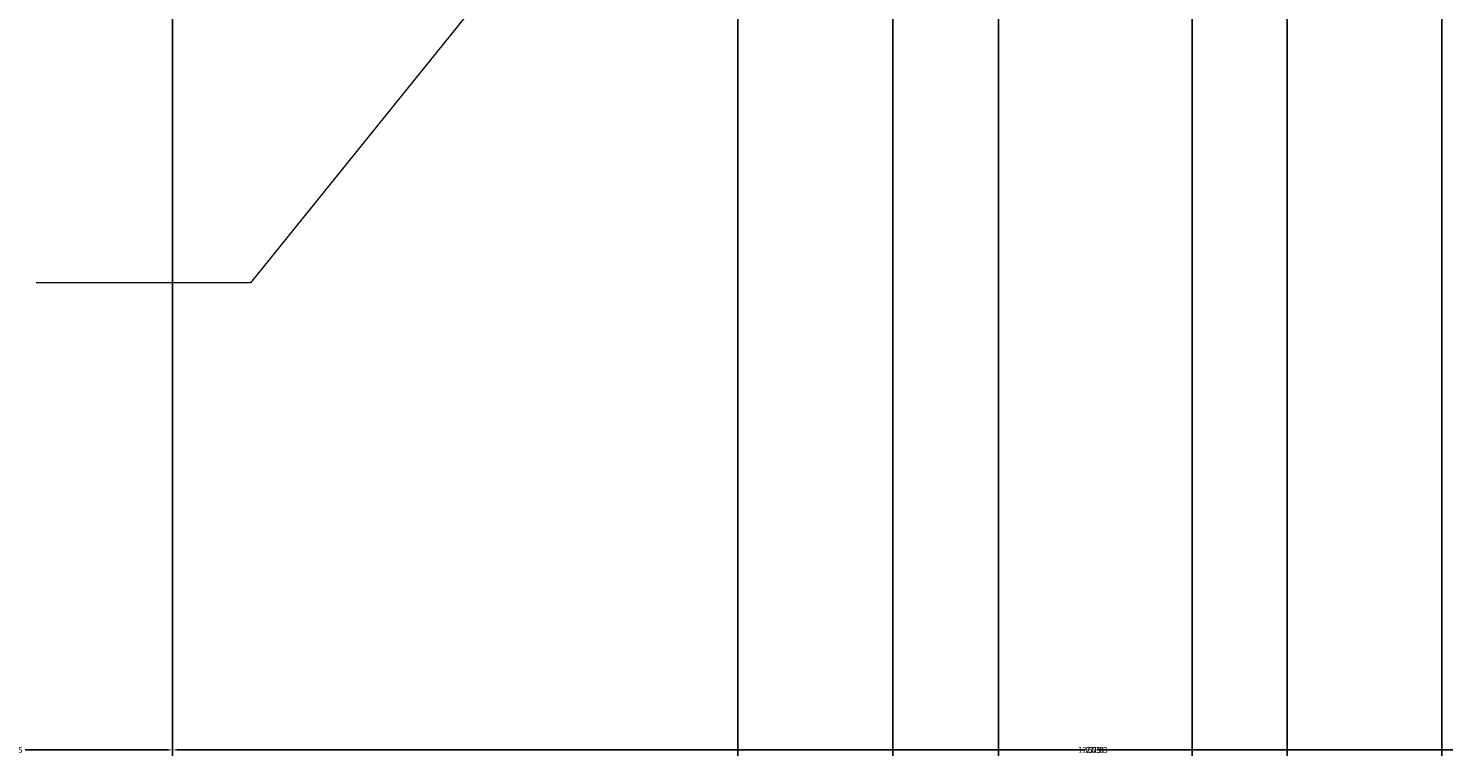
# Model space of a CAD drawing. Units: inches. Extents: x -1 to 292, y -3 to 199.
# Tile 34 of 52: x 211 to 255, y -3 to 20. Entities that reach past the tile are written whole.
import ezdxf

# ---------------------------------------------------------------- set-up
doc = ezdxf.new("R2010")
doc.units = ezdxf.units.IN
doc.header["$MEASUREMENT"] = 0
doc.layers.add('M-ANNO-LEAD', color=2, linetype='Continuous', lineweight=18)
doc.layers.add('M-DIMS', color=2, linetype='Continuous', lineweight=18)
doc.styles.get("Standard").update_dxf_attribs({"font": 'arial.ttf'})
doc.dimstyles.get("Standard").update_dxf_attribs({"dimtxt": 0.18, "dimasz": 0.18, "dimexe": 0.18, "dimexo": 0.0625, "dimgap": 0.09, "dimtad": 0, "dimtih": 1, "dimtoh": 1, "dimdec": 4, "dimzin": 0, "dimdsep": 46, "dimtxsty": 'Standard', "dimcen": 0.09, "dimadec": 0, "dimazin": 0, "dimtfac": 1, "dimtdec": 4, "dimtofl": 0, "dimtmove": 0, "dimatfit": 3, "dimfxl": 1, "dimtolj": 1, "dimtzin": 0, "dimarcsym": 0})

# ---------------------------------------------------------------- blocks, each defined once
blk = doc.blocks.new('*D24')
at = {"layer": 'Defpoints', "color": 0, "transparency": 16777216}
for p in [(215.241, 55.034), (205.115, 54.582), (215.241, -2.71)]:
    blk.add_point(p, dxfattribs=at)
at = {"layer": 'M-DIMS', "color": 0, "lineweight": -2, "transparency": 16777216}
for p, q in [((215.241, 54.971), (215.241, -2.89)), ((205.115, 54.52), (205.115, -2.89)), ((205.295, -2.71), (209.722, -2.71)), ((215.061, -2.71), (210.634, -2.71))]:
    blk.add_line(p, q, dxfattribs=at)
at = {"layer": 'M-DIMS', "color": 0, "transparency": 16777216}
for points in [[(205.295, -2.68), (205.295, -2.74), (205.115, -2.71)], [(215.061, -2.68), (215.061, -2.74), (215.241, -2.71)]]:
    blk.add_solid(points, dxfattribs=at)
at = {"layer": 'M-DIMS', "color": 0, "transparency": 16777216, "insert": (210.178, -2.71), "char_height": 0.18, "attachment_point": 5}
blk.add_mtext('\\A1;10.125', dxfattribs=at)
blk = doc.blocks.new('*D25')
at = {"layer": 'Defpoints', "color": 0, "transparency": 16777216}
for p in [(215.241, 88.13), (273.066, 88.419), (273.066, -2.71)]:
    blk.add_point(p, dxfattribs=at)
at = {"layer": 'M-DIMS', "color": 0, "lineweight": -2, "transparency": 16777216}
for p, q in [((215.241, 88.068), (215.241, -2.89)), ((273.066, 88.357), (273.066, -2.89)), ((215.421, -2.71), (243.76, -2.71)), ((272.886, -2.71), (244.547, -2.71))]:
    blk.add_line(p, q, dxfattribs=at)
at = {"layer": 'M-DIMS', "color": 0, "transparency": 16777216}
for points in [[(215.421, -2.68), (215.421, -2.74), (215.241, -2.71)], [(272.886, -2.68), (272.886, -2.74), (273.066, -2.71)]]:
    blk.add_solid(points, dxfattribs=at)
at = {"layer": 'M-DIMS', "color": 0, "transparency": 16777216, "insert": (244.153, -2.71), "char_height": 0.18, "attachment_point": 5}
blk.add_mtext('\\A1;57.83', dxfattribs=at)
blk = doc.blocks.new('*D28')
at = {"layer": 'Defpoints', "color": 0, "transparency": 16777216}
for p in [(241.044, 80.582), (247.095, 80.582), (247.095, -2.71)]:
    blk.add_point(p, dxfattribs=at)
at = {"layer": 'M-DIMS', "color": 0, "lineweight": -2, "transparency": 16777216}
for p, q in [((241.044, 80.52), (241.044, -2.89)), ((247.095, 80.52), (247.095, -2.89)), ((241.224, -2.71), (243.692, -2.71)), ((246.915, -2.71), (244.446, -2.71))]:
    blk.add_line(p, q, dxfattribs=at)
at = {"layer": 'M-DIMS', "color": 0, "transparency": 16777216}
for points in [[(241.224, -2.68), (241.224, -2.74), (241.044, -2.71)], [(246.915, -2.68), (246.915, -2.74), (247.095, -2.71)]]:
    blk.add_solid(points, dxfattribs=at)
at = {"layer": 'M-DIMS', "color": 0, "transparency": 16777216, "insert": (244.069, -2.71), "char_height": 0.18, "attachment_point": 5}
blk.add_mtext('\\A1;6.051', dxfattribs=at)
blk = doc.blocks.new('*D30')
at = {"layer": 'Defpoints', "color": 0, "transparency": 16777216}
for p in [(232.903, 62.582), (254.903, 62.582), (254.903, -2.71)]:
    blk.add_point(p, dxfattribs=at)
at = {"layer": 'M-DIMS', "color": 0, "lineweight": -2, "transparency": 16777216}
for p, q in [((232.903, 62.52), (232.903, -2.89)), ((254.903, 62.52), (254.903, -2.89)), ((233.083, -2.71), (243.684, -2.71)), ((254.723, -2.71), (244.123, -2.71))]:
    blk.add_line(p, q, dxfattribs=at)
at = {"layer": 'M-DIMS', "color": 0, "transparency": 16777216}
for points in [[(233.083, -2.68), (233.083, -2.74), (232.903, -2.71)], [(254.723, -2.68), (254.723, -2.74), (254.903, -2.71)]]:
    blk.add_solid(points, dxfattribs=at)
at = {"layer": 'M-DIMS', "color": 0, "transparency": 16777216, "insert": (243.903, -2.71), "char_height": 0.18, "attachment_point": 5}
blk.add_mtext('\\A1;22', dxfattribs=at)
blk = doc.blocks.new('*D32')
at = {"layer": 'Defpoints', "color": 0, "transparency": 16777216}
for p in [(237.744, 67.423), (250.063, 67.423), (250.063, -2.71)]:
    blk.add_point(p, dxfattribs=at)
at = {"layer": 'M-DIMS', "color": 0, "lineweight": -2, "transparency": 16777216}
for p, q in [((237.744, 67.36), (237.744, -2.89)), ((250.063, 67.36), (250.063, -2.89)), ((237.924, -2.71), (243.448, -2.71)), ((249.883, -2.71), (244.359, -2.71))]:
    blk.add_line(p, q, dxfattribs=at)
at = {"layer": 'M-DIMS', "color": 0, "transparency": 16777216}
for points in [[(237.924, -2.68), (237.924, -2.74), (237.744, -2.71)], [(249.883, -2.68), (249.883, -2.74), (250.063, -2.71)]]:
    blk.add_solid(points, dxfattribs=at)
at = {"layer": 'M-DIMS', "color": 0, "transparency": 16777216, "insert": (243.903, -2.71), "char_height": 0.18, "attachment_point": 5}
blk.add_mtext('\\A1;12.319', dxfattribs=at)

msp = doc.modelspace()

# ---------------------------------------------------------------- linework, layer by layer
at = {"layer": 'M-ANNO-LEAD'}
for p, q in [((239.9895, 39.5261), (217.6733, 11.8896)), ((217.6733, 11.8896), (210.9785, 11.8896))]:
    msp.add_line(p, q, dxfattribs=at)

# ---------------------------------------------------------------- dimensions: what is measured, and where the dimension line sits
at = {"layer": 'M-DIMS'}
for base, p1, p2, override, picture, middle in [((273.0659, -2.7104), (215.2407, 88.1304), (273.0659, 88.4191), {"dimdec": 2, "dimlfac": 1, "dimrnd": 0, "dimzin": 0, "dimdsep": 46, "dimlunit": 2}, '*D25', (244.1533, -2.7104)), ((247.0947, -2.7104), (241.0437, 80.5821), (247.0947, 80.5821), {"dimdec": 3, "dimlfac": 1, "dimrnd": 0, "dimzin": 0, "dimdsep": 46, "dimlunit": 2}, '*D28', (244.0692, -2.7104)), ((250.0626, -2.7104), (237.744, 67.4228), (250.0626, 67.4228), {"dimdec": 3, "dimlfac": 1, "dimrnd": 0, "dimzin": 0, "dimdsep": 46, "dimlunit": 2}, '*D32', (243.9033, -2.7104)), ((254.9033, -2.7104), (232.9033, 62.5821), (254.9033, 62.5821), {"dimdec": 0, "dimlfac": 1, "dimrnd": 0, "dimzin": 0, "dimdsep": 46, "dimlunit": 2}, '*D30', (243.9033, -2.7104)), ((215.2407, -2.7104), (205.1155, 54.5821), (215.2407, 55.0337), {"dimdec": 3, "dimlfac": 1, "dimrnd": 0, "dimzin": 0, "dimdsep": 46, "dimlunit": 2}, '*D24', (210.1781, -2.7104))]:
    dim = msp.add_linear_dim(base=base, p1=p1, p2=p2, dimstyle='Standard', override=override, dxfattribs=at)
    dim.commit()
    dim.dimension.update_dxf_attribs({"geometry": picture, "text_midpoint": middle})

doc.saveas('drawing.dxf')
